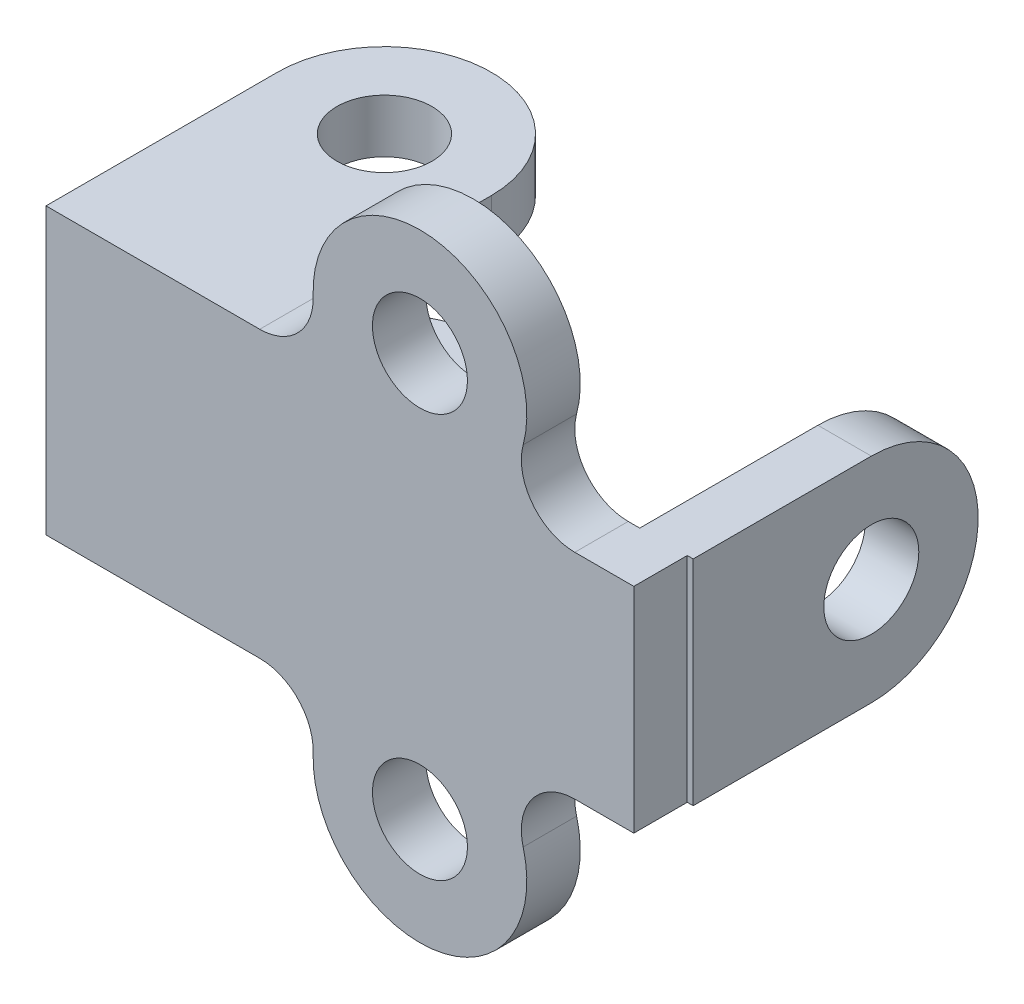
ISO-10303-21;
HEADER;
FILE_DESCRIPTION(('STEP AP214'),'2;1');
FILE_NAME('part.step','',(''),(''),'','','');
FILE_SCHEMA(('AUTOMOTIVE_DESIGN { 1 0 10303 214 1 1 1 1 }'));
ENDSEC;
DATA;
#1=APPLICATION_CONTEXT('core data for automotive mechanical design processes');
#2=APPLICATION_PROTOCOL_DEFINITION('international standard','automotive_design',2000,#1);
#3=PRODUCT_CONTEXT('',#1,'mechanical');
#4=PRODUCT('Part','Part','',(#3));
#5=PRODUCT_RELATED_PRODUCT_CATEGORY('part','',(#4));
#6=PRODUCT_DEFINITION_FORMATION('','',#4);
#7=PRODUCT_DEFINITION_CONTEXT('part definition',#1,'design');
#8=PRODUCT_DEFINITION('design','',#6,#7);
#9=PRODUCT_DEFINITION_SHAPE('','',#8);
#10=(LENGTH_UNIT() NAMED_UNIT(*) SI_UNIT(.MILLI.,.METRE.));
#11=(NAMED_UNIT(*) PLANE_ANGLE_UNIT() SI_UNIT($,.RADIAN.));
#12=(NAMED_UNIT(*) SI_UNIT($,.STERADIAN.) SOLID_ANGLE_UNIT());
#13=UNCERTAINTY_MEASURE_WITH_UNIT(LENGTH_MEASURE(1.E-05),#10,'distance_accuracy_value','');
#14=(GEOMETRIC_REPRESENTATION_CONTEXT(3) GLOBAL_UNCERTAINTY_ASSIGNED_CONTEXT((#13)) GLOBAL_UNIT_ASSIGNED_CONTEXT((#10,
#11,#12)) REPRESENTATION_CONTEXT('',''));
#15=CARTESIAN_POINT('',(0.,0.,0.));
#16=DIRECTION('',(0.,0.,1.));
#17=DIRECTION('',(1.,0.,0.));
#18=AXIS2_PLACEMENT_3D('',#15,#16,#17);
#19=CARTESIAN_POINT('',(36.,-9.,9.));
#20=DIRECTION('',(0.,0.,1.));
#21=DIRECTION('',(1.,0.,0.));
#22=AXIS2_PLACEMENT_3D('',#19,#20,#21);
#23=PLANE('',#22);
#24=CARTESIAN_POINT('',(62.9814751264641,58.,9.));
#25=DIRECTION('',(0.,0.,1.));
#26=DIRECTION('',(1.,0.,0.));
#27=AXIS2_PLACEMENT_3D('',#24,#25,#26);
#28=CIRCLE('',#27,8.);
#29=CARTESIAN_POINT('',(70.9814751264641,58.,9.));
#30=VERTEX_POINT('',#29);
#31=EDGE_CURVE('E295',#30,#30,#28,.T.);
#32=ORIENTED_EDGE('',*,*,#31,.F.);
#33=EDGE_LOOP('',(#32));
#34=FACE_BOUND('',#33,.T.);
#35=DIRECTION('',(1.,0.,0.));
#36=VECTOR('',#35,1.);
#37=CARTESIAN_POINT('',(0.,0.,9.));
#38=LINE('',#37,#36);
#39=CARTESIAN_POINT('',(0.,0.,9.));
#40=VERTEX_POINT('',#39);
#41=CARTESIAN_POINT('',(36.,0.,9.));
#42=VERTEX_POINT('',#41);
#43=EDGE_CURVE('E300',#40,#42,#38,.T.);
#44=ORIENTED_EDGE('',*,*,#43,.T.);
#45=CARTESIAN_POINT('',(36.,-9.,9.));
#46=DIRECTION('',(0.,0.,-1.));
#47=DIRECTION('',(1.,0.,0.));
#48=AXIS2_PLACEMENT_3D('',#45,#46,#47);
#49=CIRCLE('',#48,9.00000000000001);
#50=CARTESIAN_POINT('',(44.9938250421547,-9.33333333333333,9.));
#51=VERTEX_POINT('',#50);
#52=EDGE_CURVE('E304',#42,#51,#49,.T.);
#53=ORIENTED_EDGE('',*,*,#52,.T.);
#54=CARTESIAN_POINT('',(62.9814751264641,-10.,9.));
#55=DIRECTION('',(0.,0.,1.));
#56=DIRECTION('',(1.,0.,0.));
#57=AXIS2_PLACEMENT_3D('',#54,#55,#56);
#58=CIRCLE('',#57,18.);
#59=CARTESIAN_POINT('',(80.3660148736711,-5.33333333333334,9.));
#60=VERTEX_POINT('',#59);
#61=EDGE_CURVE('E303',#51,#60,#58,.T.);
#62=ORIENTED_EDGE('',*,*,#61,.T.);
#63=CARTESIAN_POINT('',(89.0582847472747,-3.00000000000001,9.));
#64=DIRECTION('',(0.,0.,-1.));
#65=DIRECTION('',(1.,0.,0.));
#66=AXIS2_PLACEMENT_3D('',#63,#64,#65);
#67=CIRCLE('',#66,9.00000000000001);
#68=CARTESIAN_POINT('',(89.0582847472747,6.,9.));
#69=VERTEX_POINT('',#68);
#70=EDGE_CURVE('E308',#60,#69,#67,.T.);
#71=ORIENTED_EDGE('',*,*,#70,.T.);
#72=DIRECTION('',(1.,0.,0.));
#73=VECTOR('',#72,1.);
#74=CARTESIAN_POINT('',(99.,6.,9.));
#75=LINE('',#74,#73);
#76=CARTESIAN_POINT('',(99.,6.,9.));
#77=VERTEX_POINT('',#76);
#78=EDGE_CURVE('E306',#69,#77,#75,.T.);
#79=ORIENTED_EDGE('',*,*,#78,.T.);
#80=DIRECTION('',(0.,1.,0.));
#81=VECTOR('',#80,1.);
#82=CARTESIAN_POINT('',(99.,24.,9.));
#83=LINE('',#82,#81);
#84=CARTESIAN_POINT('',(99.,42.,9.));
#85=VERTEX_POINT('',#84);
#86=EDGE_CURVE('E309',#77,#85,#83,.T.);
#87=ORIENTED_EDGE('',*,*,#86,.T.);
#88=DIRECTION('',(-1.,0.,0.));
#89=VECTOR('',#88,1.);
#90=CARTESIAN_POINT('',(99.,42.,9.));
#91=LINE('',#90,#89);
#92=CARTESIAN_POINT('',(89.0582847472746,42.,9.));
#93=VERTEX_POINT('',#92);
#94=EDGE_CURVE('E315',#85,#93,#91,.T.);
#95=ORIENTED_EDGE('',*,*,#94,.T.);
#96=CARTESIAN_POINT('',(89.0582847472746,51.,9.));
#97=DIRECTION('',(0.,0.,-1.));
#98=DIRECTION('',(1.,0.,0.));
#99=AXIS2_PLACEMENT_3D('',#96,#97,#98);
#100=CIRCLE('',#99,8.99999999999999);
#101=CARTESIAN_POINT('',(80.3660148736711,53.3333333333333,9.));
#102=VERTEX_POINT('',#101);
#103=EDGE_CURVE('E314',#93,#102,#100,.T.);
#104=ORIENTED_EDGE('',*,*,#103,.T.);
#105=CARTESIAN_POINT('',(62.9814751264641,58.,9.));
#106=DIRECTION('',(0.,0.,1.));
#107=DIRECTION('',(1.,0.,0.));
#108=AXIS2_PLACEMENT_3D('',#105,#106,#107);
#109=CIRCLE('',#108,18.);
#110=CARTESIAN_POINT('',(44.9938250421547,57.3333333333333,9.));
#111=VERTEX_POINT('',#110);
#112=EDGE_CURVE('E316',#102,#111,#109,.T.);
#113=ORIENTED_EDGE('',*,*,#112,.T.);
#114=CARTESIAN_POINT('',(36.,57.,9.));
#115=DIRECTION('',(0.,0.,-1.));
#116=DIRECTION('',(1.,0.,0.));
#117=AXIS2_PLACEMENT_3D('',#114,#115,#116);
#118=CIRCLE('',#117,9.);
#119=CARTESIAN_POINT('',(36.,48.,9.));
#120=VERTEX_POINT('',#119);
#121=EDGE_CURVE('E318',#111,#120,#118,.T.);
#122=ORIENTED_EDGE('',*,*,#121,.T.);
#123=DIRECTION('',(-1.,0.,0.));
#124=VECTOR('',#123,1.);
#125=CARTESIAN_POINT('',(0.,48.,9.));
#126=LINE('',#125,#124);
#127=CARTESIAN_POINT('',(0.,48.,9.));
#128=VERTEX_POINT('',#127);
#129=EDGE_CURVE('E319',#120,#128,#126,.T.);
#130=ORIENTED_EDGE('',*,*,#129,.T.);
#131=DIRECTION('',(0.,-1.,0.));
#132=VECTOR('',#131,1.);
#133=CARTESIAN_POINT('',(0.,0.,9.));
#134=LINE('',#133,#132);
#135=EDGE_CURVE('E325',#128,#40,#134,.T.);
#136=ORIENTED_EDGE('',*,*,#135,.T.);
#137=EDGE_LOOP('',(#44,#53,#62,#71,#79,#87,#95,#104,#113,#122,#130,#136));
#138=FACE_BOUND('',#137,.T.);
#139=CARTESIAN_POINT('',(62.9814751264641,-10.,9.));
#140=DIRECTION('',(0.,0.,1.));
#141=DIRECTION('',(1.,0.,0.));
#142=AXIS2_PLACEMENT_3D('',#139,#140,#141);
#143=CIRCLE('',#142,8.00000000000001);
#144=CARTESIAN_POINT('',(70.9814751264641,-10.,9.));
#145=VERTEX_POINT('',#144);
#146=EDGE_CURVE('E289',#145,#145,#143,.T.);
#147=ORIENTED_EDGE('',*,*,#146,.F.);
#148=EDGE_LOOP('',(#147));
#149=FACE_BOUND('',#148,.T.);
#150=ADVANCED_FACE('F39',(#34,#138,#149),#23,.T.);
#151=CARTESIAN_POINT('',(36.,-9.,0.));
#152=DIRECTION('',(0.,0.,1.));
#153=DIRECTION('',(1.,0.,0.));
#154=AXIS2_PLACEMENT_3D('',#151,#152,#153);
#155=PLANE('',#154);
#156=DIRECTION('',(1.,0.,0.));
#157=VECTOR('',#156,1.);
#158=CARTESIAN_POINT('',(0.,39.,0.));
#159=LINE('',#158,#157);
#160=CARTESIAN_POINT('',(0.,39.,0.));
#161=VERTEX_POINT('',#160);
#162=CARTESIAN_POINT('',(36.,39.,0.));
#163=VERTEX_POINT('',#162);
#164=EDGE_CURVE('E199',#161,#163,#159,.T.);
#165=ORIENTED_EDGE('',*,*,#164,.T.);
#166=DIRECTION('',(0.,1.,0.));
#167=VECTOR('',#166,1.);
#168=CARTESIAN_POINT('',(36.,39.,0.));
#169=LINE('',#168,#167);
#170=CARTESIAN_POINT('',(36.,48.,0.));
#171=VERTEX_POINT('',#170);
#172=EDGE_CURVE('E188',#163,#171,#169,.T.);
#173=ORIENTED_EDGE('',*,*,#172,.T.);
#174=CARTESIAN_POINT('',(36.,57.,0.));
#175=DIRECTION('',(0.,0.,-1.));
#176=DIRECTION('',(1.,0.,0.));
#177=AXIS2_PLACEMENT_3D('',#174,#175,#176);
#178=CIRCLE('',#177,9.);
#179=CARTESIAN_POINT('',(44.9938250421547,57.3333333333333,0.));
#180=VERTEX_POINT('',#179);
#181=EDGE_CURVE('E341',#180,#171,#178,.T.);
#182=ORIENTED_EDGE('',*,*,#181,.F.);
#183=CARTESIAN_POINT('',(62.9814751264641,58.,0.));
#184=DIRECTION('',(0.,0.,1.));
#185=DIRECTION('',(1.,0.,0.));
#186=AXIS2_PLACEMENT_3D('',#183,#184,#185);
#187=CIRCLE('',#186,18.);
#188=CARTESIAN_POINT('',(80.3660148736711,53.3333333333333,0.));
#189=VERTEX_POINT('',#188);
#190=EDGE_CURVE('E338',#189,#180,#187,.T.);
#191=ORIENTED_EDGE('',*,*,#190,.F.);
#192=CARTESIAN_POINT('',(89.0582847472746,51.,0.));
#193=DIRECTION('',(0.,0.,-1.));
#194=DIRECTION('',(1.,0.,0.));
#195=AXIS2_PLACEMENT_3D('',#192,#193,#194);
#196=CIRCLE('',#195,8.99999999999999);
#197=CARTESIAN_POINT('',(89.0582847472746,42.,0.));
#198=VERTEX_POINT('',#197);
#199=EDGE_CURVE('E340',#198,#189,#196,.T.);
#200=ORIENTED_EDGE('',*,*,#199,.F.);
#201=DIRECTION('',(-1.,0.,0.));
#202=VECTOR('',#201,1.);
#203=CARTESIAN_POINT('',(99.,42.,0.));
#204=LINE('',#203,#202);
#205=CARTESIAN_POINT('',(91.,42.,0.));
#206=VERTEX_POINT('',#205);
#207=EDGE_CURVE('E337',#206,#198,#204,.T.);
#208=ORIENTED_EDGE('',*,*,#207,.F.);
#209=DIRECTION('',(0.,-1.,0.));
#210=VECTOR('',#209,1.);
#211=CARTESIAN_POINT('',(91.,42.,0.));
#212=LINE('',#211,#210);
#213=CARTESIAN_POINT('',(91.,6.,0.));
#214=VERTEX_POINT('',#213);
#215=EDGE_CURVE('E262',#206,#214,#212,.T.);
#216=ORIENTED_EDGE('',*,*,#215,.T.);
#217=DIRECTION('',(1.,0.,0.));
#218=VECTOR('',#217,1.);
#219=CARTESIAN_POINT('',(99.,6.,0.));
#220=LINE('',#219,#218);
#221=CARTESIAN_POINT('',(89.0582847472747,6.,0.));
#222=VERTEX_POINT('',#221);
#223=EDGE_CURVE('E329',#222,#214,#220,.T.);
#224=ORIENTED_EDGE('',*,*,#223,.F.);
#225=CARTESIAN_POINT('',(89.0582847472747,-3.00000000000001,0.));
#226=DIRECTION('',(0.,0.,-1.));
#227=DIRECTION('',(1.,0.,0.));
#228=AXIS2_PLACEMENT_3D('',#225,#226,#227);
#229=CIRCLE('',#228,9.00000000000001);
#230=CARTESIAN_POINT('',(80.3660148736711,-5.33333333333334,0.));
#231=VERTEX_POINT('',#230);
#232=EDGE_CURVE('E327',#231,#222,#229,.T.);
#233=ORIENTED_EDGE('',*,*,#232,.F.);
#234=CARTESIAN_POINT('',(62.9814751264641,-10.,0.));
#235=DIRECTION('',(0.,0.,1.));
#236=DIRECTION('',(1.,0.,0.));
#237=AXIS2_PLACEMENT_3D('',#234,#235,#236);
#238=CIRCLE('',#237,18.);
#239=CARTESIAN_POINT('',(44.9938250421547,-9.33333333333333,0.));
#240=VERTEX_POINT('',#239);
#241=EDGE_CURVE('E326',#240,#231,#238,.T.);
#242=ORIENTED_EDGE('',*,*,#241,.F.);
#243=CARTESIAN_POINT('',(36.,-9.,0.));
#244=DIRECTION('',(0.,0.,-1.));
#245=DIRECTION('',(1.,0.,0.));
#246=AXIS2_PLACEMENT_3D('',#243,#244,#245);
#247=CIRCLE('',#246,9.00000000000001);
#248=CARTESIAN_POINT('',(36.,0.,0.));
#249=VERTEX_POINT('',#248);
#250=EDGE_CURVE('E293',#249,#240,#247,.T.);
#251=ORIENTED_EDGE('',*,*,#250,.F.);
#252=DIRECTION('',(0.,-1.,0.));
#253=VECTOR('',#252,1.);
#254=CARTESIAN_POINT('',(36.,9.,0.));
#255=LINE('',#254,#253);
#256=CARTESIAN_POINT('',(36.,9.,0.));
#257=VERTEX_POINT('',#256);
#258=EDGE_CURVE('E243',#257,#249,#255,.T.);
#259=ORIENTED_EDGE('',*,*,#258,.F.);
#260=DIRECTION('',(1.,0.,0.));
#261=VECTOR('',#260,1.);
#262=CARTESIAN_POINT('',(0.,9.,0.));
#263=LINE('',#262,#261);
#264=CARTESIAN_POINT('',(0.,9.,0.));
#265=VERTEX_POINT('',#264);
#266=EDGE_CURVE('E232',#265,#257,#263,.T.);
#267=ORIENTED_EDGE('',*,*,#266,.F.);
#268=DIRECTION('',(0.,-1.,0.));
#269=VECTOR('',#268,1.);
#270=CARTESIAN_POINT('',(0.,0.,0.));
#271=LINE('',#270,#269);
#272=EDGE_CURVE('E301',#161,#265,#271,.T.);
#273=ORIENTED_EDGE('',*,*,#272,.F.);
#274=EDGE_LOOP('',(#165,#173,#182,#191,#200,#208,#216,#224,#233,#242,#251,#259,#267,#273));
#275=FACE_BOUND('',#274,.T.);
#276=CARTESIAN_POINT('',(62.9814751264641,58.,0.));
#277=DIRECTION('',(0.,0.,1.));
#278=DIRECTION('',(1.,0.,0.));
#279=AXIS2_PLACEMENT_3D('',#276,#277,#278);
#280=CIRCLE('',#279,8.);
#281=CARTESIAN_POINT('',(70.9814751264641,58.,0.));
#282=VERTEX_POINT('',#281);
#283=EDGE_CURVE('E288',#282,#282,#280,.T.);
#284=ORIENTED_EDGE('',*,*,#283,.T.);
#285=EDGE_LOOP('',(#284));
#286=FACE_BOUND('',#285,.T.);
#287=CARTESIAN_POINT('',(62.9814751264641,-10.,0.));
#288=DIRECTION('',(0.,0.,1.));
#289=DIRECTION('',(1.,0.,0.));
#290=AXIS2_PLACEMENT_3D('',#287,#288,#289);
#291=CIRCLE('',#290,8.00000000000001);
#292=CARTESIAN_POINT('',(70.9814751264641,-10.,0.));
#293=VERTEX_POINT('',#292);
#294=EDGE_CURVE('E278',#293,#293,#291,.T.);
#295=ORIENTED_EDGE('',*,*,#294,.T.);
#296=EDGE_LOOP('',(#295));
#297=FACE_BOUND('',#296,.T.);
#298=ADVANCED_FACE('F385',(#275,#286,#297),#155,.F.);
#299=CARTESIAN_POINT('',(0.,0.,9.));
#300=DIRECTION('',(0.,1.,0.));
#301=DIRECTION('',(0.,0.,1.));
#302=AXIS2_PLACEMENT_3D('',#299,#300,#301);
#303=PLANE('',#302);
#304=DIRECTION('',(0.,0.,-1.));
#305=VECTOR('',#304,1.);
#306=CARTESIAN_POINT('',(0.,0.,9.));
#307=LINE('',#306,#305);
#308=CARTESIAN_POINT('',(0.,0.,-30.));
#309=VERTEX_POINT('',#308);
#310=EDGE_CURVE('E322',#40,#309,#307,.T.);
#311=ORIENTED_EDGE('',*,*,#310,.T.);
#312=CARTESIAN_POINT('',(18.,0.,-30.));
#313=DIRECTION('',(0.,1.,0.));
#314=DIRECTION('',(0.,0.,1.));
#315=AXIS2_PLACEMENT_3D('',#312,#313,#314);
#316=CIRCLE('',#315,18.);
#317=CARTESIAN_POINT('',(36.,0.,-30.));
#318=VERTEX_POINT('',#317);
#319=EDGE_CURVE('E223',#318,#309,#316,.T.);
#320=ORIENTED_EDGE('',*,*,#319,.F.);
#321=DIRECTION('',(0.,0.,-1.));
#322=VECTOR('',#321,1.);
#323=CARTESIAN_POINT('',(36.,0.,0.));
#324=LINE('',#323,#322);
#325=EDGE_CURVE('E231',#249,#318,#324,.T.);
#326=ORIENTED_EDGE('',*,*,#325,.F.);
#327=DIRECTION('',(0.,0.,-1.));
#328=VECTOR('',#327,1.);
#329=CARTESIAN_POINT('',(36.,0.,9.));
#330=LINE('',#329,#328);
#331=EDGE_CURVE('E11',#42,#249,#330,.T.);
#332=ORIENTED_EDGE('',*,*,#331,.F.);
#333=ORIENTED_EDGE('',*,*,#43,.F.);
#334=EDGE_LOOP('',(#311,#320,#326,#332,#333));
#335=FACE_BOUND('',#334,.T.);
#336=CARTESIAN_POINT('',(18.,0.,-30.));
#337=DIRECTION('',(0.,1.,0.));
#338=DIRECTION('',(0.,0.,1.));
#339=AXIS2_PLACEMENT_3D('',#336,#337,#338);
#340=CIRCLE('',#339,8.);
#341=CARTESIAN_POINT('',(18.,0.,-22.));
#342=VERTEX_POINT('',#341);
#343=EDGE_CURVE('E218',#342,#342,#340,.T.);
#344=ORIENTED_EDGE('',*,*,#343,.T.);
#345=EDGE_LOOP('',(#344));
#346=FACE_BOUND('',#345,.T.);
#347=ADVANCED_FACE('F41',(#335,#346),#303,.F.);
#348=CARTESIAN_POINT('',(36.,-9.,9.));
#349=DIRECTION('',(0.,0.,-1.));
#350=DIRECTION('',(-1.,0.,0.));
#351=AXIS2_PLACEMENT_3D('',#348,#349,#350);
#352=CYLINDRICAL_SURFACE('',#351,9.00000000000001);
#353=ORIENTED_EDGE('',*,*,#250,.T.);
#354=DIRECTION('',(0.,0.,-1.));
#355=VECTOR('',#354,1.);
#356=CARTESIAN_POINT('',(44.9938250421547,-9.33333333333333,9.));
#357=LINE('',#356,#355);
#358=EDGE_CURVE('E50',#51,#240,#357,.T.);
#359=ORIENTED_EDGE('',*,*,#358,.F.);
#360=ORIENTED_EDGE('',*,*,#52,.F.);
#361=ORIENTED_EDGE('',*,*,#331,.T.);
#362=EDGE_LOOP('',(#353,#359,#360,#361));
#363=FACE_BOUND('',#362,.T.);
#364=ADVANCED_FACE('F402',(#363),#352,.F.);
#365=CARTESIAN_POINT('',(62.9814751264641,-10.,9.));
#366=DIRECTION('',(0.,0.,-1.));
#367=DIRECTION('',(-1.,0.,0.));
#368=AXIS2_PLACEMENT_3D('',#365,#366,#367);
#369=CYLINDRICAL_SURFACE('',#368,18.);
#370=ORIENTED_EDGE('',*,*,#241,.T.);
#371=DIRECTION('',(0.,0.,-1.));
#372=VECTOR('',#371,1.);
#373=CARTESIAN_POINT('',(80.3660148736711,-5.33333333333334,9.));
#374=LINE('',#373,#372);
#375=EDGE_CURVE('E369',#60,#231,#374,.T.);
#376=ORIENTED_EDGE('',*,*,#375,.F.);
#377=ORIENTED_EDGE('',*,*,#61,.F.);
#378=ORIENTED_EDGE('',*,*,#358,.T.);
#379=EDGE_LOOP('',(#370,#376,#377,#378));
#380=FACE_BOUND('',#379,.T.);
#381=ADVANCED_FACE('F376',(#380),#369,.T.);
#382=CARTESIAN_POINT('',(89.0582847472747,-3.00000000000001,9.));
#383=DIRECTION('',(0.,0.,-1.));
#384=DIRECTION('',(-1.,0.,0.));
#385=AXIS2_PLACEMENT_3D('',#382,#383,#384);
#386=CYLINDRICAL_SURFACE('',#385,9.00000000000001);
#387=ORIENTED_EDGE('',*,*,#232,.T.);
#388=DIRECTION('',(0.,0.,-1.));
#389=VECTOR('',#388,1.);
#390=CARTESIAN_POINT('',(89.0582847472747,6.,9.));
#391=LINE('',#390,#389);
#392=EDGE_CURVE('E368',#69,#222,#391,.T.);
#393=ORIENTED_EDGE('',*,*,#392,.F.);
#394=ORIENTED_EDGE('',*,*,#70,.F.);
#395=ORIENTED_EDGE('',*,*,#375,.T.);
#396=EDGE_LOOP('',(#387,#393,#394,#395));
#397=FACE_BOUND('',#396,.T.);
#398=ADVANCED_FACE('F389',(#397),#386,.F.);
#399=CARTESIAN_POINT('',(99.,6.,9.));
#400=DIRECTION('',(0.,1.,0.));
#401=DIRECTION('',(-1.,0.,0.));
#402=AXIS2_PLACEMENT_3D('',#399,#400,#401);
#403=PLANE('',#402);
#404=ORIENTED_EDGE('',*,*,#223,.T.);
#405=DIRECTION('',(0.,0.,-1.));
#406=VECTOR('',#405,1.);
#407=CARTESIAN_POINT('',(91.,6.,0.));
#408=LINE('',#407,#406);
#409=CARTESIAN_POINT('',(91.,5.99999999999999,-30.));
#410=VERTEX_POINT('',#409);
#411=EDGE_CURVE('E64',#214,#410,#408,.T.);
#412=ORIENTED_EDGE('',*,*,#411,.T.);
#413=DIRECTION('',(1.,0.,0.));
#414=VECTOR('',#413,1.);
#415=CARTESIAN_POINT('',(91.,5.99999999999999,-30.));
#416=LINE('',#415,#414);
#417=CARTESIAN_POINT('',(100.,5.99999999999999,-30.));
#418=VERTEX_POINT('',#417);
#419=EDGE_CURVE('E279',#410,#418,#416,.T.);
#420=ORIENTED_EDGE('',*,*,#419,.T.);
#421=DIRECTION('',(0.,0.,-1.));
#422=VECTOR('',#421,1.);
#423=CARTESIAN_POINT('',(100.,6.,0.));
#424=LINE('',#423,#422);
#425=CARTESIAN_POINT('',(100.,6.,0.));
#426=VERTEX_POINT('',#425);
#427=EDGE_CURVE('E261',#426,#418,#424,.T.);
#428=ORIENTED_EDGE('',*,*,#427,.F.);
#429=DIRECTION('',(1.,0.,0.));
#430=VECTOR('',#429,1.);
#431=CARTESIAN_POINT('',(91.,6.,0.));
#432=LINE('',#431,#430);
#433=CARTESIAN_POINT('',(99.,6.,0.));
#434=VERTEX_POINT('',#433);
#435=EDGE_CURVE('E282',#434,#426,#432,.T.);
#436=ORIENTED_EDGE('',*,*,#435,.F.);
#437=DIRECTION('',(0.,0.,-1.));
#438=VECTOR('',#437,1.);
#439=CARTESIAN_POINT('',(99.,6.,9.));
#440=LINE('',#439,#438);
#441=EDGE_CURVE('E361',#77,#434,#440,.T.);
#442=ORIENTED_EDGE('',*,*,#441,.F.);
#443=ORIENTED_EDGE('',*,*,#78,.F.);
#444=ORIENTED_EDGE('',*,*,#392,.T.);
#445=EDGE_LOOP('',(#404,#412,#420,#428,#436,#442,#443,#444));
#446=FACE_BOUND('',#445,.T.);
#447=ADVANCED_FACE('F394',(#446),#403,.F.);
#448=CARTESIAN_POINT('',(99.,24.,9.));
#449=DIRECTION('',(-1.,0.,0.));
#450=DIRECTION('',(0.,0.,1.));
#451=AXIS2_PLACEMENT_3D('',#448,#449,#450);
#452=PLANE('',#451);
#453=DIRECTION('',(0.,1.,0.));
#454=VECTOR('',#453,1.);
#455=CARTESIAN_POINT('',(99.,24.,0.));
#456=LINE('',#455,#454);
#457=CARTESIAN_POINT('',(99.,42.,0.));
#458=VERTEX_POINT('',#457);
#459=EDGE_CURVE('E334',#434,#458,#456,.T.);
#460=ORIENTED_EDGE('',*,*,#459,.T.);
#461=DIRECTION('',(0.,0.,-1.));
#462=VECTOR('',#461,1.);
#463=CARTESIAN_POINT('',(99.,42.,9.));
#464=LINE('',#463,#462);
#465=EDGE_CURVE('E357',#85,#458,#464,.T.);
#466=ORIENTED_EDGE('',*,*,#465,.F.);
#467=ORIENTED_EDGE('',*,*,#86,.F.);
#468=ORIENTED_EDGE('',*,*,#441,.T.);
#469=EDGE_LOOP('',(#460,#466,#467,#468));
#470=FACE_BOUND('',#469,.T.);
#471=ADVANCED_FACE('F456',(#470),#452,.F.);
#472=CARTESIAN_POINT('',(99.,42.,9.));
#473=DIRECTION('',(0.,-1.,0.));
#474=DIRECTION('',(0.,0.,-1.));
#475=AXIS2_PLACEMENT_3D('',#472,#473,#474);
#476=PLANE('',#475);
#477=ORIENTED_EDGE('',*,*,#465,.T.);
#478=DIRECTION('',(1.,0.,0.));
#479=VECTOR('',#478,1.);
#480=CARTESIAN_POINT('',(91.,42.,0.));
#481=LINE('',#480,#479);
#482=CARTESIAN_POINT('',(100.,42.,0.));
#483=VERTEX_POINT('',#482);
#484=EDGE_CURVE('E285',#458,#483,#481,.T.);
#485=ORIENTED_EDGE('',*,*,#484,.T.);
#486=DIRECTION('',(0.,0.,1.));
#487=VECTOR('',#486,1.);
#488=CARTESIAN_POINT('',(100.,42.,-30.));
#489=LINE('',#488,#487);
#490=CARTESIAN_POINT('',(100.,42.,-30.));
#491=VERTEX_POINT('',#490);
#492=EDGE_CURVE('E269',#491,#483,#489,.T.);
#493=ORIENTED_EDGE('',*,*,#492,.F.);
#494=DIRECTION('',(1.,0.,0.));
#495=VECTOR('',#494,1.);
#496=CARTESIAN_POINT('',(91.,42.,-30.));
#497=LINE('',#496,#495);
#498=CARTESIAN_POINT('',(91.,42.,-30.));
#499=VERTEX_POINT('',#498);
#500=EDGE_CURVE('E270',#499,#491,#497,.T.);
#501=ORIENTED_EDGE('',*,*,#500,.F.);
#502=DIRECTION('',(0.,0.,1.));
#503=VECTOR('',#502,1.);
#504=CARTESIAN_POINT('',(91.,42.,-30.));
#505=LINE('',#504,#503);
#506=EDGE_CURVE('E257',#499,#206,#505,.T.);
#507=ORIENTED_EDGE('',*,*,#506,.T.);
#508=ORIENTED_EDGE('',*,*,#207,.T.);
#509=DIRECTION('',(0.,0.,-1.));
#510=VECTOR('',#509,1.);
#511=CARTESIAN_POINT('',(89.0582847472746,42.,9.));
#512=LINE('',#511,#510);
#513=EDGE_CURVE('E356',#93,#198,#512,.T.);
#514=ORIENTED_EDGE('',*,*,#513,.F.);
#515=ORIENTED_EDGE('',*,*,#94,.F.);
#516=EDGE_LOOP('',(#477,#485,#493,#501,#507,#508,#514,#515));
#517=FACE_BOUND('',#516,.T.);
#518=ADVANCED_FACE('F441',(#517),#476,.F.);
#519=CARTESIAN_POINT('',(89.0582847472746,51.,9.));
#520=DIRECTION('',(0.,0.,-1.));
#521=DIRECTION('',(-1.,0.,0.));
#522=AXIS2_PLACEMENT_3D('',#519,#520,#521);
#523=CYLINDRICAL_SURFACE('',#522,8.99999999999999);
#524=ORIENTED_EDGE('',*,*,#199,.T.);
#525=DIRECTION('',(0.,0.,-1.));
#526=VECTOR('',#525,1.);
#527=CARTESIAN_POINT('',(80.3660148736711,53.3333333333333,9.));
#528=LINE('',#527,#526);
#529=EDGE_CURVE('E351',#102,#189,#528,.T.);
#530=ORIENTED_EDGE('',*,*,#529,.F.);
#531=ORIENTED_EDGE('',*,*,#103,.F.);
#532=ORIENTED_EDGE('',*,*,#513,.T.);
#533=EDGE_LOOP('',(#524,#530,#531,#532));
#534=FACE_BOUND('',#533,.T.);
#535=ADVANCED_FACE('F438',(#534),#523,.F.);
#536=CARTESIAN_POINT('',(62.9814751264641,58.,9.));
#537=DIRECTION('',(0.,0.,-1.));
#538=DIRECTION('',(-1.,0.,0.));
#539=AXIS2_PLACEMENT_3D('',#536,#537,#538);
#540=CYLINDRICAL_SURFACE('',#539,18.);
#541=ORIENTED_EDGE('',*,*,#190,.T.);
#542=DIRECTION('',(0.,0.,-1.));
#543=VECTOR('',#542,1.);
#544=CARTESIAN_POINT('',(44.9938250421547,57.3333333333333,9.));
#545=LINE('',#544,#543);
#546=EDGE_CURVE('E352',#111,#180,#545,.T.);
#547=ORIENTED_EDGE('',*,*,#546,.F.);
#548=ORIENTED_EDGE('',*,*,#112,.F.);
#549=ORIENTED_EDGE('',*,*,#529,.T.);
#550=EDGE_LOOP('',(#541,#547,#548,#549));
#551=FACE_BOUND('',#550,.T.);
#552=ADVANCED_FACE('F432',(#551),#540,.T.);
#553=CARTESIAN_POINT('',(36.,57.,9.));
#554=DIRECTION('',(0.,0.,-1.));
#555=DIRECTION('',(-1.,0.,0.));
#556=AXIS2_PLACEMENT_3D('',#553,#554,#555);
#557=CYLINDRICAL_SURFACE('',#556,9.);
#558=ORIENTED_EDGE('',*,*,#181,.T.);
#559=DIRECTION('',(0.,0.,-1.));
#560=VECTOR('',#559,1.);
#561=CARTESIAN_POINT('',(36.,48.,9.));
#562=LINE('',#561,#560);
#563=EDGE_CURVE('E346',#120,#171,#562,.T.);
#564=ORIENTED_EDGE('',*,*,#563,.F.);
#565=ORIENTED_EDGE('',*,*,#121,.F.);
#566=ORIENTED_EDGE('',*,*,#546,.T.);
#567=EDGE_LOOP('',(#558,#564,#565,#566));
#568=FACE_BOUND('',#567,.T.);
#569=ADVANCED_FACE('F429',(#568),#557,.F.);
#570=CARTESIAN_POINT('',(0.,48.,9.));
#571=DIRECTION('',(0.,-1.,0.));
#572=DIRECTION('',(1.,0.,0.));
#573=AXIS2_PLACEMENT_3D('',#570,#571,#572);
#574=PLANE('',#573);
#575=ORIENTED_EDGE('',*,*,#563,.T.);
#576=DIRECTION('',(0.,0.,-1.));
#577=VECTOR('',#576,1.);
#578=CARTESIAN_POINT('',(36.,48.,0.));
#579=LINE('',#578,#577);
#580=CARTESIAN_POINT('',(36.,48.,-30.));
#581=VERTEX_POINT('',#580);
#582=EDGE_CURVE('E202',#171,#581,#579,.T.);
#583=ORIENTED_EDGE('',*,*,#582,.T.);
#584=CARTESIAN_POINT('',(18.,48.,-30.));
#585=DIRECTION('',(0.,1.,0.));
#586=DIRECTION('',(0.,0.,1.));
#587=AXIS2_PLACEMENT_3D('',#584,#585,#586);
#588=CIRCLE('',#587,18.);
#589=CARTESIAN_POINT('',(0.,48.,-30.));
#590=VERTEX_POINT('',#589);
#591=EDGE_CURVE('E208',#581,#590,#588,.T.);
#592=ORIENTED_EDGE('',*,*,#591,.T.);
#593=DIRECTION('',(0.,0.,-1.));
#594=VECTOR('',#593,1.);
#595=CARTESIAN_POINT('',(0.,48.,9.));
#596=LINE('',#595,#594);
#597=EDGE_CURVE('E183',#128,#590,#596,.T.);
#598=ORIENTED_EDGE('',*,*,#597,.F.);
#599=ORIENTED_EDGE('',*,*,#129,.F.);
#600=EDGE_LOOP('',(#575,#583,#592,#598,#599));
#601=FACE_BOUND('',#600,.T.);
#602=CARTESIAN_POINT('',(18.,48.,-30.));
#603=DIRECTION('',(0.,1.,0.));
#604=DIRECTION('',(0.,0.,1.));
#605=AXIS2_PLACEMENT_3D('',#602,#603,#604);
#606=CIRCLE('',#605,8.);
#607=CARTESIAN_POINT('',(18.,48.,-22.));
#608=VERTEX_POINT('',#607);
#609=EDGE_CURVE('E211',#608,#608,#606,.T.);
#610=ORIENTED_EDGE('',*,*,#609,.F.);
#611=EDGE_LOOP('',(#610));
#612=FACE_BOUND('',#611,.T.);
#613=ADVANCED_FACE('F421',(#601,#612),#574,.F.);
#614=CARTESIAN_POINT('',(0.,0.,9.));
#615=DIRECTION('',(1.,0.,0.));
#616=DIRECTION('',(0.,0.,-1.));
#617=AXIS2_PLACEMENT_3D('',#614,#615,#616);
#618=PLANE('',#617);
#619=ORIENTED_EDGE('',*,*,#597,.T.);
#620=DIRECTION('',(0.,1.,0.));
#621=VECTOR('',#620,1.);
#622=CARTESIAN_POINT('',(0.,39.,-30.));
#623=LINE('',#622,#621);
#624=CARTESIAN_POINT('',(0.,39.,-30.));
#625=VERTEX_POINT('',#624);
#626=EDGE_CURVE('E182',#625,#590,#623,.T.);
#627=ORIENTED_EDGE('',*,*,#626,.F.);
#628=DIRECTION('',(0.,0.,1.));
#629=VECTOR('',#628,1.);
#630=CARTESIAN_POINT('',(0.,39.,-30.));
#631=LINE('',#630,#629);
#632=EDGE_CURVE('E53',#625,#161,#631,.T.);
#633=ORIENTED_EDGE('',*,*,#632,.T.);
#634=ORIENTED_EDGE('',*,*,#272,.T.);
#635=DIRECTION('',(0.,0.,1.));
#636=VECTOR('',#635,1.);
#637=CARTESIAN_POINT('',(0.,9.,-30.));
#638=LINE('',#637,#636);
#639=CARTESIAN_POINT('',(0.,9.,-30.));
#640=VERTEX_POINT('',#639);
#641=EDGE_CURVE('E234',#640,#265,#638,.T.);
#642=ORIENTED_EDGE('',*,*,#641,.F.);
#643=DIRECTION('',(0.,-1.,0.));
#644=VECTOR('',#643,1.);
#645=CARTESIAN_POINT('',(0.,9.,-30.));
#646=LINE('',#645,#644);
#647=EDGE_CURVE('E246',#640,#309,#646,.T.);
#648=ORIENTED_EDGE('',*,*,#647,.T.);
#649=ORIENTED_EDGE('',*,*,#310,.F.);
#650=ORIENTED_EDGE('',*,*,#135,.F.);
#651=EDGE_LOOP('',(#619,#627,#633,#634,#642,#648,#649,#650));
#652=FACE_BOUND('',#651,.T.);
#653=ADVANCED_FACE('F185',(#652),#618,.F.);
#654=CARTESIAN_POINT('',(62.9814751264641,58.,9.));
#655=DIRECTION('',(0.,0.,-1.));
#656=DIRECTION('',(-1.,0.,0.));
#657=AXIS2_PLACEMENT_3D('',#654,#655,#656);
#658=CYLINDRICAL_SURFACE('',#657,8.);
#659=ORIENTED_EDGE('',*,*,#31,.T.);
#660=EDGE_LOOP('',(#659));
#661=FACE_BOUND('',#660,.T.);
#662=ORIENTED_EDGE('',*,*,#283,.F.);
#663=EDGE_LOOP('',(#662));
#664=FACE_BOUND('',#663,.T.);
#665=ADVANCED_FACE('F480',(#661,#664),#658,.F.);
#666=CARTESIAN_POINT('',(62.9814751264641,-10.,9.));
#667=DIRECTION('',(0.,0.,-1.));
#668=DIRECTION('',(-1.,0.,0.));
#669=AXIS2_PLACEMENT_3D('',#666,#667,#668);
#670=CYLINDRICAL_SURFACE('',#669,8.00000000000001);
#671=ORIENTED_EDGE('',*,*,#146,.T.);
#672=EDGE_LOOP('',(#671));
#673=FACE_BOUND('',#672,.T.);
#674=ORIENTED_EDGE('',*,*,#294,.F.);
#675=EDGE_LOOP('',(#674));
#676=FACE_BOUND('',#675,.T.);
#677=ADVANCED_FACE('F510',(#673,#676),#670,.F.);
#678=CARTESIAN_POINT('',(91.,42.,0.));
#679=DIRECTION('',(0.,0.,1.));
#680=DIRECTION('',(1.,0.,0.));
#681=AXIS2_PLACEMENT_3D('',#678,#679,#680);
#682=PLANE('',#681);
#683=ORIENTED_EDGE('',*,*,#459,.F.);
#684=ORIENTED_EDGE('',*,*,#435,.T.);
#685=DIRECTION('',(0.,-1.,0.));
#686=VECTOR('',#685,1.);
#687=CARTESIAN_POINT('',(100.,42.,0.));
#688=LINE('',#687,#686);
#689=EDGE_CURVE('E272',#483,#426,#688,.T.);
#690=ORIENTED_EDGE('',*,*,#689,.F.);
#691=ORIENTED_EDGE('',*,*,#484,.F.);
#692=EDGE_LOOP('',(#683,#684,#690,#691));
#693=FACE_BOUND('',#692,.T.);
#694=ADVANCED_FACE('F457',(#693),#682,.T.);
#695=CARTESIAN_POINT('',(91.,24.,-30.));
#696=DIRECTION('',(1.,0.,0.));
#697=DIRECTION('',(0.,0.,-1.));
#698=AXIS2_PLACEMENT_3D('',#695,#696,#697);
#699=CYLINDRICAL_SURFACE('',#698,18.);
#700=CARTESIAN_POINT('',(100.,24.,-30.));
#701=DIRECTION('',(1.,0.,0.));
#702=DIRECTION('',(0.,0.,-1.));
#703=AXIS2_PLACEMENT_3D('',#700,#701,#702);
#704=CIRCLE('',#703,18.);
#705=EDGE_CURVE('E255',#418,#491,#704,.T.);
#706=ORIENTED_EDGE('',*,*,#705,.F.);
#707=ORIENTED_EDGE('',*,*,#419,.F.);
#708=CARTESIAN_POINT('',(91.,24.,-30.));
#709=DIRECTION('',(1.,0.,0.));
#710=DIRECTION('',(0.,0.,-1.));
#711=AXIS2_PLACEMENT_3D('',#708,#709,#710);
#712=CIRCLE('',#711,18.);
#713=EDGE_CURVE('E260',#410,#499,#712,.T.);
#714=ORIENTED_EDGE('',*,*,#713,.T.);
#715=ORIENTED_EDGE('',*,*,#500,.T.);
#716=EDGE_LOOP('',(#706,#707,#714,#715));
#717=FACE_BOUND('',#716,.T.);
#718=ADVANCED_FACE('F448',(#717),#699,.T.);
#719=CARTESIAN_POINT('',(91.,24.,-30.));
#720=DIRECTION('',(1.,0.,0.));
#721=DIRECTION('',(0.,0.,-1.));
#722=AXIS2_PLACEMENT_3D('',#719,#720,#721);
#723=PLANE('',#722);
#724=CARTESIAN_POINT('',(91.,24.,-30.));
#725=DIRECTION('',(1.,0.,0.));
#726=DIRECTION('',(0.,0.,-1.));
#727=AXIS2_PLACEMENT_3D('',#724,#725,#726);
#728=CIRCLE('',#727,8.);
#729=CARTESIAN_POINT('',(91.,24.,-38.));
#730=VERTEX_POINT('',#729);
#731=EDGE_CURVE('E253',#730,#730,#728,.T.);
#732=ORIENTED_EDGE('',*,*,#731,.T.);
#733=EDGE_LOOP('',(#732));
#734=FACE_BOUND('',#733,.T.);
#735=ORIENTED_EDGE('',*,*,#713,.F.);
#736=ORIENTED_EDGE('',*,*,#411,.F.);
#737=ORIENTED_EDGE('',*,*,#215,.F.);
#738=ORIENTED_EDGE('',*,*,#506,.F.);
#739=EDGE_LOOP('',(#735,#736,#737,#738));
#740=FACE_BOUND('',#739,.T.);
#741=ADVANCED_FACE('F449',(#734,#740),#723,.F.);
#742=CARTESIAN_POINT('',(100.,24.,-30.));
#743=DIRECTION('',(1.,0.,0.));
#744=DIRECTION('',(0.,0.,-1.));
#745=AXIS2_PLACEMENT_3D('',#742,#743,#744);
#746=PLANE('',#745);
#747=CARTESIAN_POINT('',(100.,24.,-30.));
#748=DIRECTION('',(1.,0.,0.));
#749=DIRECTION('',(0.,0.,-1.));
#750=AXIS2_PLACEMENT_3D('',#747,#748,#749);
#751=CIRCLE('',#750,8.);
#752=CARTESIAN_POINT('',(100.,24.,-38.));
#753=VERTEX_POINT('',#752);
#754=EDGE_CURVE('E247',#753,#753,#751,.T.);
#755=ORIENTED_EDGE('',*,*,#754,.F.);
#756=EDGE_LOOP('',(#755));
#757=FACE_BOUND('',#756,.T.);
#758=ORIENTED_EDGE('',*,*,#705,.T.);
#759=ORIENTED_EDGE('',*,*,#492,.T.);
#760=ORIENTED_EDGE('',*,*,#689,.T.);
#761=ORIENTED_EDGE('',*,*,#427,.T.);
#762=EDGE_LOOP('',(#758,#759,#760,#761));
#763=FACE_BOUND('',#762,.T.);
#764=ADVANCED_FACE('F455',(#757,#763),#746,.T.);
#765=CARTESIAN_POINT('',(91.,24.,-30.));
#766=DIRECTION('',(1.,0.,0.));
#767=DIRECTION('',(0.,0.,-1.));
#768=AXIS2_PLACEMENT_3D('',#765,#766,#767);
#769=CYLINDRICAL_SURFACE('',#768,8.);
#770=ORIENTED_EDGE('',*,*,#731,.F.);
#771=EDGE_LOOP('',(#770));
#772=FACE_BOUND('',#771,.T.);
#773=ORIENTED_EDGE('',*,*,#754,.T.);
#774=EDGE_LOOP('',(#773));
#775=FACE_BOUND('',#774,.T.);
#776=ADVANCED_FACE('F570',(#772,#775),#769,.F.);
#777=CARTESIAN_POINT('',(18.,9.,-30.));
#778=DIRECTION('',(0.,1.,0.));
#779=DIRECTION('',(0.,0.,1.));
#780=AXIS2_PLACEMENT_3D('',#777,#778,#779);
#781=PLANE('',#780);
#782=CARTESIAN_POINT('',(18.,9.,-30.));
#783=DIRECTION('',(0.,1.,0.));
#784=DIRECTION('',(0.,0.,1.));
#785=AXIS2_PLACEMENT_3D('',#782,#783,#784);
#786=CIRCLE('',#785,18.);
#787=CARTESIAN_POINT('',(36.,9.,-30.));
#788=VERTEX_POINT('',#787);
#789=EDGE_CURVE('E230',#788,#640,#786,.T.);
#790=ORIENTED_EDGE('',*,*,#789,.T.);
#791=ORIENTED_EDGE('',*,*,#641,.T.);
#792=ORIENTED_EDGE('',*,*,#266,.T.);
#793=DIRECTION('',(0.,0.,-1.));
#794=VECTOR('',#793,1.);
#795=CARTESIAN_POINT('',(36.,9.,0.));
#796=LINE('',#795,#794);
#797=EDGE_CURVE('E240',#257,#788,#796,.T.);
#798=ORIENTED_EDGE('',*,*,#797,.T.);
#799=EDGE_LOOP('',(#790,#791,#792,#798));
#800=FACE_BOUND('',#799,.T.);
#801=CARTESIAN_POINT('',(18.,9.,-30.));
#802=DIRECTION('',(0.,1.,0.));
#803=DIRECTION('',(0.,0.,1.));
#804=AXIS2_PLACEMENT_3D('',#801,#802,#803);
#805=CIRCLE('',#804,8.);
#806=CARTESIAN_POINT('',(18.,9.,-22.));
#807=VERTEX_POINT('',#806);
#808=EDGE_CURVE('E225',#807,#807,#805,.T.);
#809=ORIENTED_EDGE('',*,*,#808,.F.);
#810=EDGE_LOOP('',(#809));
#811=FACE_BOUND('',#810,.T.);
#812=ADVANCED_FACE('F412',(#800,#811),#781,.T.);
#813=CARTESIAN_POINT('',(18.,9.,-30.));
#814=DIRECTION('',(0.,-1.,0.));
#815=DIRECTION('',(0.,0.,-1.));
#816=AXIS2_PLACEMENT_3D('',#813,#814,#815);
#817=CYLINDRICAL_SURFACE('',#816,18.);
#818=ORIENTED_EDGE('',*,*,#319,.T.);
#819=ORIENTED_EDGE('',*,*,#647,.F.);
#820=ORIENTED_EDGE('',*,*,#789,.F.);
#821=DIRECTION('',(0.,-1.,0.));
#822=VECTOR('',#821,1.);
#823=CARTESIAN_POINT('',(36.,9.,-30.));
#824=LINE('',#823,#822);
#825=EDGE_CURVE('E239',#788,#318,#824,.T.);
#826=ORIENTED_EDGE('',*,*,#825,.T.);
#827=EDGE_LOOP('',(#818,#819,#820,#826));
#828=FACE_BOUND('',#827,.T.);
#829=ADVANCED_FACE('F411',(#828),#817,.T.);
#830=CARTESIAN_POINT('',(36.,9.,0.));
#831=DIRECTION('',(-1.,0.,0.));
#832=DIRECTION('',(0.,0.,1.));
#833=AXIS2_PLACEMENT_3D('',#830,#831,#832);
#834=PLANE('',#833);
#835=ORIENTED_EDGE('',*,*,#325,.T.);
#836=ORIENTED_EDGE('',*,*,#825,.F.);
#837=ORIENTED_EDGE('',*,*,#797,.F.);
#838=ORIENTED_EDGE('',*,*,#258,.T.);
#839=EDGE_LOOP('',(#835,#836,#837,#838));
#840=FACE_BOUND('',#839,.T.);
#841=ADVANCED_FACE('F410',(#840),#834,.F.);
#842=CARTESIAN_POINT('',(18.,9.,-30.));
#843=DIRECTION('',(0.,-1.,0.));
#844=DIRECTION('',(0.,0.,-1.));
#845=AXIS2_PLACEMENT_3D('',#842,#843,#844);
#846=CYLINDRICAL_SURFACE('',#845,8.);
#847=ORIENTED_EDGE('',*,*,#808,.T.);
#848=EDGE_LOOP('',(#847));
#849=FACE_BOUND('',#848,.T.);
#850=ORIENTED_EDGE('',*,*,#343,.F.);
#851=EDGE_LOOP('',(#850));
#852=FACE_BOUND('',#851,.T.);
#853=ADVANCED_FACE('F627',(#849,#852),#846,.F.);
#854=CARTESIAN_POINT('',(18.,39.,-30.));
#855=DIRECTION('',(0.,1.,0.));
#856=DIRECTION('',(0.,0.,1.));
#857=AXIS2_PLACEMENT_3D('',#854,#855,#856);
#858=CYLINDRICAL_SURFACE('',#857,18.);
#859=ORIENTED_EDGE('',*,*,#591,.F.);
#860=DIRECTION('',(0.,1.,0.));
#861=VECTOR('',#860,1.);
#862=CARTESIAN_POINT('',(36.,39.,-30.));
#863=LINE('',#862,#861);
#864=CARTESIAN_POINT('',(36.,39.,-30.));
#865=VERTEX_POINT('',#864);
#866=EDGE_CURVE('E204',#865,#581,#863,.T.);
#867=ORIENTED_EDGE('',*,*,#866,.F.);
#868=CARTESIAN_POINT('',(18.,39.,-30.));
#869=DIRECTION('',(0.,1.,0.));
#870=DIRECTION('',(0.,0.,1.));
#871=AXIS2_PLACEMENT_3D('',#868,#869,#870);
#872=CIRCLE('',#871,18.);
#873=EDGE_CURVE('E197',#865,#625,#872,.T.);
#874=ORIENTED_EDGE('',*,*,#873,.T.);
#875=ORIENTED_EDGE('',*,*,#626,.T.);
#876=EDGE_LOOP('',(#859,#867,#874,#875));
#877=FACE_BOUND('',#876,.T.);
#878=ADVANCED_FACE('F201',(#877),#858,.T.);
#879=CARTESIAN_POINT('',(36.,39.,0.));
#880=DIRECTION('',(1.,0.,0.));
#881=DIRECTION('',(0.,0.,-1.));
#882=AXIS2_PLACEMENT_3D('',#879,#880,#881);
#883=PLANE('',#882);
#884=ORIENTED_EDGE('',*,*,#582,.F.);
#885=ORIENTED_EDGE('',*,*,#172,.F.);
#886=DIRECTION('',(0.,0.,-1.));
#887=VECTOR('',#886,1.);
#888=CARTESIAN_POINT('',(36.,39.,0.));
#889=LINE('',#888,#887);
#890=EDGE_CURVE('E194',#163,#865,#889,.T.);
#891=ORIENTED_EDGE('',*,*,#890,.T.);
#892=ORIENTED_EDGE('',*,*,#866,.T.);
#893=EDGE_LOOP('',(#884,#885,#891,#892));
#894=FACE_BOUND('',#893,.T.);
#895=ADVANCED_FACE('F426',(#894),#883,.T.);
#896=CARTESIAN_POINT('',(18.,39.,-30.));
#897=DIRECTION('',(0.,1.,0.));
#898=DIRECTION('',(0.,0.,1.));
#899=AXIS2_PLACEMENT_3D('',#896,#897,#898);
#900=PLANE('',#899);
#901=CARTESIAN_POINT('',(18.,39.,-30.));
#902=DIRECTION('',(0.,1.,0.));
#903=DIRECTION('',(0.,0.,1.));
#904=AXIS2_PLACEMENT_3D('',#901,#902,#903);
#905=CIRCLE('',#904,8.);
#906=CARTESIAN_POINT('',(18.,39.,-22.));
#907=VERTEX_POINT('',#906);
#908=EDGE_CURVE('E216',#907,#907,#905,.T.);
#909=ORIENTED_EDGE('',*,*,#908,.T.);
#910=EDGE_LOOP('',(#909));
#911=FACE_BOUND('',#910,.T.);
#912=ORIENTED_EDGE('',*,*,#873,.F.);
#913=ORIENTED_EDGE('',*,*,#890,.F.);
#914=ORIENTED_EDGE('',*,*,#164,.F.);
#915=ORIENTED_EDGE('',*,*,#632,.F.);
#916=EDGE_LOOP('',(#912,#913,#914,#915));
#917=FACE_BOUND('',#916,.T.);
#918=ADVANCED_FACE('F192',(#911,#917),#900,.F.);
#919=CARTESIAN_POINT('',(18.,39.,-30.));
#920=DIRECTION('',(0.,1.,0.));
#921=DIRECTION('',(0.,0.,1.));
#922=AXIS2_PLACEMENT_3D('',#919,#920,#921);
#923=CYLINDRICAL_SURFACE('',#922,8.);
#924=ORIENTED_EDGE('',*,*,#908,.F.);
#925=EDGE_LOOP('',(#924));
#926=FACE_BOUND('',#925,.T.);
#927=ORIENTED_EDGE('',*,*,#609,.T.);
#928=EDGE_LOOP('',(#927));
#929=FACE_BOUND('',#928,.T.);
#930=ADVANCED_FACE('F664',(#926,#929),#923,.F.);
#931=CLOSED_SHELL('',(#150,#298,#347,#364,#381,#398,#447,#471,#518,#535,#552,#569,#613,#653,
#665,#677,#694,#718,#741,#764,#776,#812,#829,#841,#853,#878,#895,#918,#930));
#932=MANIFOLD_SOLID_BREP('B2',#931);
#933=ADVANCED_BREP_SHAPE_REPRESENTATION('',(#18,#932),#14);
#934=SHAPE_DEFINITION_REPRESENTATION(#9,#933);
ENDSEC;
END-ISO-10303-21;
